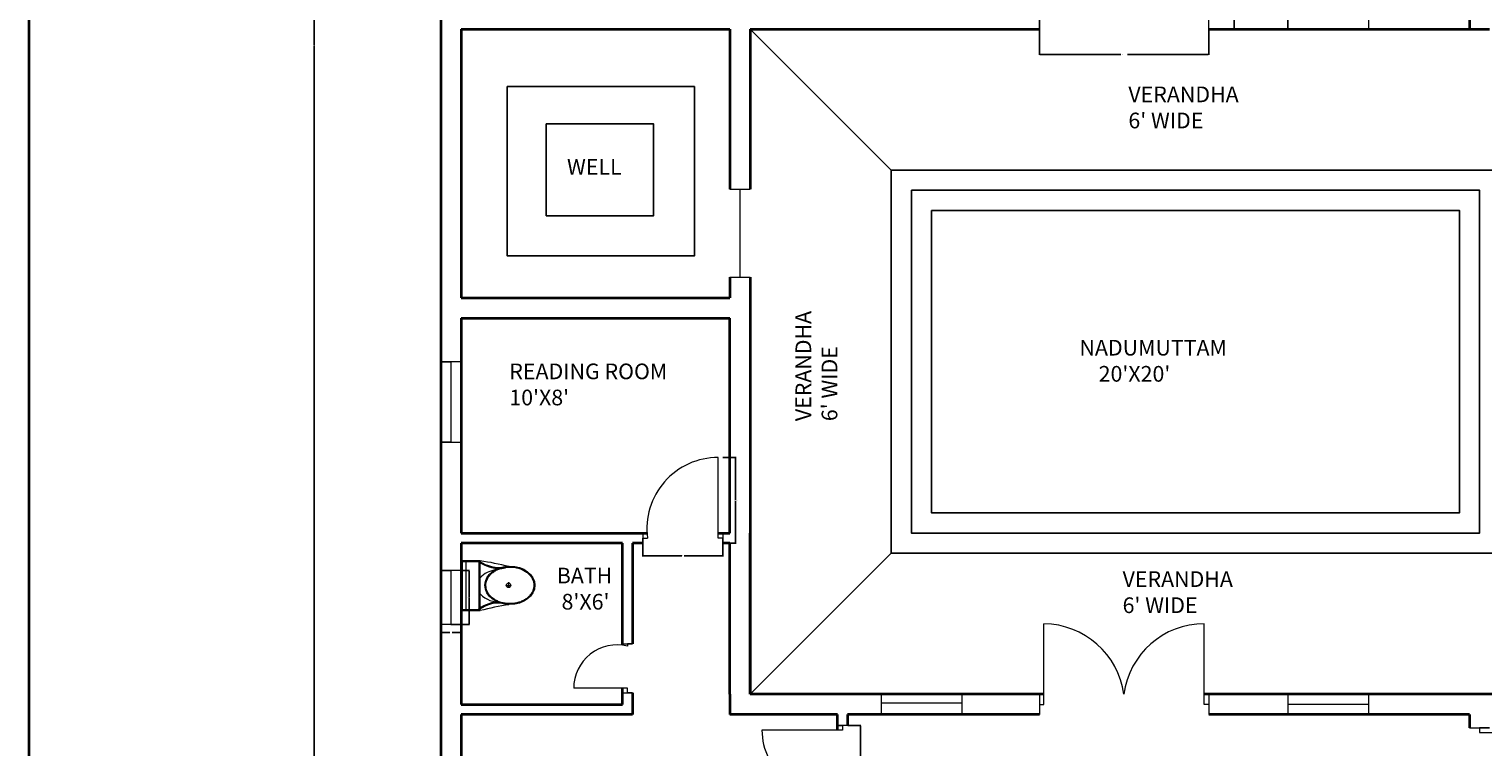
# Model space of a CAD drawing. Units: inches. Extents: x 2185 to 4426, y 1138 to 3073.
# Tile 3 of 14: x 2185 to 2834, y 1514 to 1834. Entities that reach past the tile are written whole.
import ezdxf

# ---------------------------------------------------------------- set-up
doc = ezdxf.new("R2010")
doc.units = ezdxf.units.IN
for name, color, linetype, lineweight in [('A-ANNO-DIMS', 2, 'Continuous', 18), ('A-ANNO-TTLB', 7, 'Continuous', 35), ('A-AREA-IDEN', 7, 'Continuous', 18), ('A-DOOR', 3, 'Continuous', 18), ('A-FLOR-EDGE', 7, 'Continuous', 25), ('A-FLOR-FIXT', 9, 'Continuous', 18), ('A-GLAZ', 4, 'Continuous', 18), ('A-SITE-WELL', 7, 'Continuous', 25), ('A-WALL', 7, 'Continuous', 35)]:
    doc.layers.add(name, color=color, linetype=linetype, lineweight=lineweight)
doc.styles.get("Standard").update_dxf_attribs({"font": 'arial.ttf'})
doc.dimstyles.get("Standard").update_dxf_attribs({"dimtxt": 0.18, "dimasz": 0.18, "dimexe": 0.18, "dimexo": 0.0625, "dimgap": 0.09, "dimtad": 0, "dimtih": 1, "dimtoh": 1, "dimdec": 4, "dimzin": 0, "dimdsep": 46, "dimtxsty": 'Standard', "dimcen": 0.09, "dimadec": 0, "dimazin": 0, "dimtfac": 1, "dimtdec": 4, "dimtofl": 0, "dimtmove": 0, "dimatfit": 3, "dimfxl": 1, "dimtolj": 1, "dimtzin": 0, "dimarcsym": 0})

# ---------------------------------------------------------------- blocks, each defined once
blk = doc.blocks.new('A$C31115884')
for p, q in [((283, 498), (223, 498)), ((258, 466), (258, 523)), ((0, 200), (0, 0)), ((520, 200), (0, 200)), ((10, 190), (10, 10)), ((510, 190), (10, 190)), ((510, 10), (510, 190)), ((520, 0), (520, 200)), ((510, 54), (0, 54)), ((10, 10), (510, 10)), ((0, 0), (520, 0))]:
    blk.add_line(p, q)
blk.add_circle((256, 496), 23.6)
for centre, radius, start, end in [((2778, -205), 2807, 165.4549, 171.7133), ((-295, 403), 365, 324.2091, 9.3499), ((-295, 403), 375, 324.2091, 9.3499), ((806, 403), 365, 170.6501, 215.7909), ((3237, 905), 2807, 188.2867, 194.5451), ((384, 406), 293, 190.2774, 224.1564), ((139, 406), 293, 315.8436, 2.6563), ((806, 403), 375, 179.2036, 215.7909)]:
    blk.add_arc(centre, radius, start, end)
blk.add_ellipse((256, 510), major_axis=(0, -261), ratio=0.772727)
blk.add_open_spline([(256, 259), (263, 259), (270, 260), (288, 262), (299, 265), (320, 273), (330, 278), (350, 291), (360, 299), (378, 316), (386, 326), (402, 347), (409, 358), (421, 383), (427, 395), (436, 422), (440, 436), (445, 465), (447, 480), (448, 509), (448, 524), (445, 553), (443, 568), (436, 596), (432, 610), (422, 636), (416, 649), (402, 672), (395, 683), (379, 703), (370, 712), (351, 728), (341, 735), (321, 746), (310, 751), (289, 757), (278, 759), (256, 761), (245, 761), (223, 757), (212, 754), (191, 746), (181, 741), (161, 728), (151, 720), (133, 703), (125, 693), (110, 672), (103, 660), (90, 636), (85, 623), (76, 596), (72, 582), (67, 553), (66, 538), (64, 509), (65, 494), (68, 465), (70, 450), (77, 422), (81, 408), (91, 382), (97, 370), (111, 346), (118, 335), (135, 316), (144, 307), (162, 291), (172, 284), (193, 273), (203, 269), (225, 262), (236, 260), (250, 259), (253, 259), (256, 259)], degree=3, knots=[0, 0, 0, 0, 0.110105, 0.110105, 0.285049, 0.285049, 0.459994, 0.459994, 0.634938, 0.634938, 0.809882, 0.809882, 0.984827, 0.984827, 1.159771, 1.159771, 1.334715, 1.334715, 1.50966, 1.50966, 1.684604, 1.684604, 1.859549, 1.859549, 2.034493, 2.034493, 2.209437, 2.209437, 2.384382, 2.384382, 2.559326, 2.559326, 2.73427, 2.73427, 2.909215, 2.909215, 3.084159, 3.084159, 3.259103, 3.259103, 3.434048, 3.434048, 3.608992, 3.608992, 3.783936, 3.783936, 3.958881, 3.958881, 4.133825, 4.133825, 4.30877, 4.30877, 4.483714, 4.483714, 4.658658, 4.658658, 4.833603, 4.833603, 5.008547, 5.008547, 5.183491, 5.183491, 5.358436, 5.358436, 5.53338, 5.53338, 5.708324, 5.708324, 5.883269, 5.883269, 6.058213, 6.058213, 6.233158, 6.233158, 6.283185, 6.283185, 6.283185, 6.283185])
blk = doc.blocks.new('DOOR-SGL-24-BATH-W')
for p, q in [((21.75, 21.83), (26.25, 21.83)), ((26.25, 21.83), (24, 21.83)), ((24, 21.83), (24, 20.83)), ((24, 2), (0, 2)), ((24, 0), (24, 2)), ((21.75, 0), (26.25, 0)), ((26.25, 0), (24, 0))]:
    blk.add_line(p, q)
blk.add_arc((19.38, 2), 19.38, 76.22605, 180)
blk = doc.blocks.new('DOOR-SGL-36-READING')
for p, q in [((33.62, 2.25), (33.62, 38.25)), ((0, 4.5), (0, 0)), ((0, 0), (0, 2.25)), ((0, 2.25), (2, 2.25)), ((35.62, 2.25), (33.62, 2.25)), ((35.62, 4.5), (35.62, 0)), ((35.62, 0), (35.62, 2.25))]:
    blk.add_line(p, q)
blk.add_arc((33.62, 6.36), 31.89, 90, 187.40318)
blk = doc.blocks.new('DOOR-PAIR-36-DINING')
for p, q in [((2, 4.5), (2, 40.5)), ((73.51, 4.5), (73.51, 40.5)), ((0, 9), (0, 0)), ((75.51, 0), (75.51, 9)), ((75.51, 9), (75.51, 4.5)), ((0, 0), (0, 4.5)), ((0, 4.5), (2, 4.5)), ((75.51, 4.5), (73.51, 4.5))]:
    blk.add_line(p, q)
for centre, radius, start, end in [((2, 3.7), 36.8, 8.27614, 90), ((74.14, 4.5), 36.01, 90.99344, 172.82033)]:
    blk.add_arc(centre, radius, start, end)
blk = doc.blocks.new('DOOR-SGL-36-BED-SW')
for p, q in [((36, 29.13), (0, 29.13)), ((38.25, 31.13), (33.75, 31.13)), ((33.75, 31.13), (36, 31.13)), ((36, 31.13), (36, 29.13)), ((36, 0), (36, 2)), ((33.75, 0), (38.25, 0)), ((38.25, 0), (36, 0))]:
    blk.add_line(p, q)
blk.add_arc((28.22, 29.13), 28.22, 180, 285.9925)
blk = doc.blocks.new('DOOR-PAIR-36-VERANDA')
for p, q in [((2, 4.5), (2, 40.5)), ((73.51, 4.5), (73.51, 40.5)), ((0, 9), (0, 0)), ((75.51, 9), (75.51, 0)), ((0, 4.5), (2, 4.5)), ((75.51, 4.5), (73.51, 4.5))]:
    blk.add_line(p, q)
for centre, radius, start, end in [((1.42, 3.87), 36.64, 8.05449, 89.09279), ((73.51, 4.39), 36.11, 90, 172.66346)]:
    blk.add_arc(centre, radius, start, end)
blk = doc.blocks.new('DOOR-SGL-36-BED-S')
for p, q in [((0, 31.73), (9, 31.73)), ((9, 31.73), (4.5, 31.73)), ((4.5, 31.73), (4.5, 31.73)), ((4.5, 31.73), (4.5, 29.73)), ((4.5, 29.73), (40.5, 29.73)), ((0, 0), (9, 0)), ((4.5, 0), (4.5, 2)), ((9, 0), (4.5, 0))]:
    blk.add_line(p, q)
blk.add_arc((11.82, 29.73), 28.68, 255.21093, 0)
blk = doc.blocks.new('WIN-PLAN-24IN-02')
for p, q in [((9, 24), (0, 24)), ((0, 24), (4.5, 24)), ((4.5, 24), (4.5, 0)), ((9, 0), (0, 0)), ((0, 0), (0, 0)), ((4.5, 0), (9, 0))]:
    blk.add_line(p, q)
blk = doc.blocks.new('WIN-PLAN-36IN-01')
for p, q in [((0, 9), (0, 0)), ((36, 4.5), (36, 9)), ((36, 9), (36, 0)), ((0, 0), (0, 4.5)), ((0, 4.5), (0, 4.5)), ((0, 4.5), (36, 4.5))]:
    blk.add_line(p, q)
blk = doc.blocks.new('WIN-PLAN-36IN-03')
for p, q in [((9, 36), (0, 36)), ((0, 36), (0, 36)), ((0, 36), (4.5, 36)), ((4.5, 36), (4.5, 0)), ((4.5, 0), (0, 0)), ((0, 0), (9, 0)), ((9, 0), (9, 0))]:
    blk.add_line(p, q)
blk = doc.blocks.new('WIN-PLAN-36IN-06')
for p, q in [((0, 9), (0, 0)), ((36, 9), (36, 0)), ((0, 5.12), (36, 5.12)), ((36, 5.12), (36, 5.12))]:
    blk.add_line(p, q)
blk = doc.blocks.new('WIN-PLAN-36IN-07')
for p, q in [((0, 9), (0, 0)), ((36, 9), (36, 0)), ((36, 4.5), (0, 4.5))]:
    blk.add_line(p, q)
blk = doc.blocks.new('WIN-PLAN-39IN')
for p, q in [((0, 39.26), (9, 39.26)), ((4.5, 0), (4.5, 39.26)), ((0, 0), (9, 0))]:
    blk.add_line(p, q)
blk = doc.blocks.new('WELL-PLAN')
for points in [[(0, 75.64), (83.5, 75.64), (83.5, 0), (0, 0)], [(17.44, 59), (65.29, 59), (65.29, 18), (17.44, 18)]]:
    blk.add_lwpolyline(points, close=True)
blk = doc.blocks.new('*D74')
at = {"layer": 'A-ANNO-DIMS', "color": 0, "lineweight": -2, "transparency": 16777216}
for p, q in [((2494.37, 1643.13), (2500.22, 1643.13)), ((2500.04, 1642.95), (2500.04, 1624.19)), ((2500.04, 1605.06), (2500.04, 1623.82)), ((2494.37, 1604.88), (2500.22, 1604.88))]:
    blk.add_line(p, q, dxfattribs=at)
at = {"layer": 'A-ANNO-DIMS', "color": 0, "transparency": 16777216}
for points in [[(2500.01, 1642.95), (2500.07, 1642.95), (2500.04, 1643.13)], [(2500.01, 1605.06), (2500.07, 1605.06), (2500.04, 1604.88)]]:
    blk.add_solid(points, dxfattribs=at)
at = {"layer": 'Defpoints', "color": 0, "transparency": 16777216}
for p in [(2494.31, 1643.13), (2500.04, 1643.13), (2494.31, 1604.88)]:
    blk.add_point(p, dxfattribs=at)
at = {"layer": 'A-ANNO-DIMS', "color": 0, "transparency": 16777216, "insert": (2500.04, 1624), "char_height": 0.18, "attachment_point": 5}
blk.add_mtext('\\A1;DOOR 38 TYP.', dxfattribs=at)
blk = doc.blocks.new('*D75')
at = {"layer": 'A-ANNO-DIMS', "color": 0, "lineweight": -2, "transparency": 16777216}
for p, q in [((2458.68, 1604.81), (2458.68, 1598.96)), ((2494.31, 1604.81), (2494.31, 1598.96)), ((2458.86, 1599.14), (2475.97, 1599.14)), ((2494.13, 1599.14), (2477.02, 1599.14))]:
    blk.add_line(p, q, dxfattribs=at)
at = {"layer": 'A-ANNO-DIMS', "color": 0, "transparency": 16777216}
for points in [[(2458.86, 1599.17), (2458.86, 1599.11), (2458.68, 1599.14)], [(2494.13, 1599.17), (2494.13, 1599.11), (2494.31, 1599.14)]]:
    blk.add_solid(points, dxfattribs=at)
at = {"layer": 'Defpoints', "color": 0, "transparency": 16777216}
for p in [(2458.68, 1604.88), (2494.31, 1604.88), (2494.31, 1599.14)]:
    blk.add_point(p, dxfattribs=at)
at = {"layer": 'A-ANNO-DIMS', "color": 0, "transparency": 16777216, "insert": (2476.49, 1599.14), "char_height": 0.18, "attachment_point": 5}
blk.add_mtext('\\A1;36 TYP.', dxfattribs=at)
blk = doc.blocks.new('*D76')
at = {"layer": 'A-ANNO-DIMS', "color": 0, "lineweight": -2, "transparency": 16777216}
for p, q in [((2635.64, 1834.31), (2635.64, 1822.87)), ((2711.16, 1834.31), (2711.16, 1822.87)), ((2635.82, 1823.05), (2671.91, 1823.05)), ((2710.98, 1823.05), (2674.89, 1823.05))]:
    blk.add_line(p, q, dxfattribs=at)
at = {"layer": 'A-ANNO-DIMS', "color": 0, "transparency": 16777216}
for points in [[(2635.82, 1823.08), (2635.82, 1823.02), (2635.64, 1823.05)], [(2710.98, 1823.08), (2710.98, 1823.02), (2711.16, 1823.05)]]:
    blk.add_solid(points, dxfattribs=at)
at = {"layer": 'Defpoints', "color": 0, "transparency": 16777216}
for p in [(2635.64, 1834.38), (2711.16, 1834.38), (2711.16, 1823.05)]:
    blk.add_point(p, dxfattribs=at)
at = {"layer": 'A-ANNO-DIMS', "color": 0, "transparency": 16777216, "insert": (2673.4, 1823.05), "char_height": 0.18, "attachment_point": 5}
blk.add_mtext('\\A1;DINING DOORS 76 TYP.', dxfattribs=at)
blk = doc.blocks.new('*D77')
at = {"layer": 'A-ANNO-DIMS', "color": 0, "lineweight": -2, "transparency": 16777216}
for p, q in [((2711.22, 1874.88), (2722.66, 1874.88)), ((2722.48, 1874.7), (2722.48, 1854.81)), ((2722.48, 1834.56), (2722.48, 1854.45)), ((2711.22, 1834.38), (2722.66, 1834.38))]:
    blk.add_line(p, q, dxfattribs=at)
at = {"layer": 'A-ANNO-DIMS', "color": 0, "transparency": 16777216}
for points in [[(2722.45, 1874.7), (2722.51, 1874.7), (2722.48, 1874.88)], [(2722.45, 1834.56), (2722.51, 1834.56), (2722.48, 1834.38)]]:
    blk.add_solid(points, dxfattribs=at)
at = {"layer": 'Defpoints', "color": 0, "transparency": 16777216}
for p in [(2711.16, 1874.88), (2722.48, 1874.88), (2711.16, 1834.38)]:
    blk.add_point(p, dxfattribs=at)
at = {"layer": 'A-ANNO-DIMS', "color": 0, "transparency": 16777216, "insert": (2722.48, 1854.63), "char_height": 0.18, "attachment_point": 5}
blk.add_mtext('\\A1;41 TYP.', dxfattribs=at)
blk = doc.blocks.new('*D81')
at = {"layer": 'A-ANNO-DIMS', "color": 0, "lineweight": -2, "transparency": 16777216}
for p, q in [((2550.08, 1523.44), (2555.94, 1523.44)), ((2555.76, 1523.26), (2555.76, 1507.83)), ((2555.76, 1492.05), (2555.76, 1507.47)), ((2550.08, 1491.87), (2555.94, 1491.87))]:
    blk.add_line(p, q, dxfattribs=at)
at = {"layer": 'A-ANNO-DIMS', "color": 0, "transparency": 16777216}
for points in [[(2555.73, 1523.26), (2555.79, 1523.26), (2555.76, 1523.44)], [(2555.73, 1492.05), (2555.79, 1492.05), (2555.76, 1491.87)]]:
    blk.add_solid(points, dxfattribs=at)
at = {"layer": 'Defpoints', "color": 0, "transparency": 16777216}
for p in [(2550.02, 1523.44), (2555.76, 1523.44), (2550.02, 1491.87)]:
    blk.add_point(p, dxfattribs=at)
at = {"layer": 'A-ANNO-DIMS', "color": 0, "transparency": 16777216, "insert": (2555.76, 1507.65), "char_height": 0.18, "attachment_point": 5}
blk.add_mtext('\\A1;32 TYP.', dxfattribs=at)
blk = doc.blocks.new('*D92')
at = {"layer": 'A-ANNO-DIMS', "color": 0, "lineweight": -2, "transparency": 16777216}
for p, q in [((2377.58, 1592.58), (2381.3, 1592.58)), ((2381.12, 1592.4), (2381.12, 1580.77)), ((2381.12, 1568.76), (2381.12, 1580.4)), ((2377.58, 1568.58), (2381.3, 1568.58))]:
    blk.add_line(p, q, dxfattribs=at)
at = {"layer": 'A-ANNO-DIMS', "color": 0, "transparency": 16777216}
for points in [[(2381.09, 1592.4), (2381.15, 1592.4), (2381.12, 1592.58)], [(2381.09, 1568.76), (2381.15, 1568.76), (2381.12, 1568.58)]]:
    blk.add_solid(points, dxfattribs=at)
at = {"layer": 'Defpoints', "color": 0, "transparency": 16777216}
for p in [(2377.52, 1592.58), (2381.12, 1592.58), (2377.52, 1568.58)]:
    blk.add_point(p, dxfattribs=at)
at = {"layer": 'A-ANNO-DIMS', "color": 0, "transparency": 16777216, "insert": (2381.12, 1580.58), "char_height": 0.18, "attachment_point": 5}
blk.add_mtext('\\A1;WINDOW 24 TYP.', dxfattribs=at)
blk = doc.blocks.new('*D93')
at = {"layer": 'A-ANNO-DIMS', "color": 0, "lineweight": -2, "transparency": 16777216}
for p, q in [((2368.52, 1568.52), (2368.52, 1564.8)), ((2368.7, 1564.98), (2372.56, 1564.98)), ((2377.34, 1564.98), (2373.48, 1564.98)), ((2377.52, 1568.52), (2377.52, 1564.8))]:
    blk.add_line(p, q, dxfattribs=at)
at = {"layer": 'A-ANNO-DIMS', "color": 0, "transparency": 16777216}
for points in [[(2368.7, 1565.01), (2368.7, 1564.95), (2368.52, 1564.98)], [(2377.34, 1565.01), (2377.34, 1564.95), (2377.52, 1564.98)]]:
    blk.add_solid(points, dxfattribs=at)
at = {"layer": 'Defpoints', "color": 0, "transparency": 16777216}
for p in [(2368.52, 1568.58), (2377.52, 1568.58), (2377.52, 1564.98)]:
    blk.add_point(p, dxfattribs=at)
at = {"layer": 'A-ANNO-DIMS', "color": 0, "transparency": 16777216, "insert": (2373.02, 1564.98), "char_height": 0.18, "attachment_point": 5}
blk.add_mtext('\\A1;9 TYP.', dxfattribs=at)
blk = doc.blocks.new('*D139')
at = {"layer": 'A-ANNO-DIMS', "color": 0, "lineweight": -2, "transparency": 16777216}
for p, q in [((2368.46, 2326.38), (2311.84, 2326.38)), ((2312.02, 2326.2), (2312.02, 1827.06)), ((2312.02, 1327.56), (2312.02, 1826.7)), ((2368.46, 1327.38), (2311.84, 1327.38))]:
    blk.add_line(p, q, dxfattribs=at)
at = {"layer": 'A-ANNO-DIMS', "color": 0, "transparency": 16777216}
for points in [[(2311.99, 2326.2), (2312.05, 2326.2), (2312.02, 2326.38)], [(2311.99, 1327.56), (2312.05, 1327.56), (2312.02, 1327.38)]]:
    blk.add_solid(points, dxfattribs=at)
at = {"layer": 'Defpoints', "color": 0, "transparency": 16777216}
for p in [(2312.02, 2326.38), (2368.52, 2326.38), (2368.52, 1327.38)]:
    blk.add_point(p, dxfattribs=at)
at = {"layer": 'A-ANNO-DIMS', "color": 0, "transparency": 16777216, "insert": (2312.02, 1826.88), "char_height": 0.18, "attachment_point": 5}
blk.add_mtext('\\A1;999', dxfattribs=at)

msp = doc.modelspace()

# ---------------------------------------------------------------- linework, layer by layer
at = {"layer": 'A-ANNO-TTLB'}
msp.add_lwpolyline([(2184.741, 3073.364), (4426.252, 3073.364), (4426.252, 1137.99), (2184.741, 1137.99)], close=True, dxfattribs=at)
at = {"layer": 'A-FLOR-EDGE'}
for p, q in [((2569.478, 1771.377), (2506.519, 1834.377)), ((2832.019, 1762.377), (2578.478, 1762.377)), ((2578.478, 1762.377), (2578.478, 1609.377)), ((2832.019, 1609.377), (2832.019, 1762.377)), ((2578.478, 1609.377), (2832.019, 1609.377)), ((2569.478, 1600.377), (2506.519, 1537.377))]:
    msp.add_line(p, q, dxfattribs=at)
for points in [[(2569.478, 1771.377), (2841.019, 1771.377), (2841.019, 1600.377), (2569.478, 1600.377)], [(2578.478, 1762.377), (2832.019, 1762.377), (2832.019, 1609.377), (2578.478, 1609.377)], [(2587.478, 1753.377), (2823.019, 1753.377), (2823.019, 1618.377), (2587.478, 1618.377)]]:
    msp.add_lwpolyline(points, close=True, dxfattribs=at)
at = {"layer": 'A-WALL'}
for p, q in [((2368.519, 2136.303), (2368.519, 1327.377)), ((2368.519, 2136.303), (2368.519, 1327.377)), ((2827.519, 1843.377), (2827.519, 1834.377)), ((2377.519, 1834.377), (2497.519, 1834.377)), ((2377.519, 1834.377), (2377.519, 1714.377)), ((2497.519, 1834.377), (2497.519, 1762.843)), ((2506.519, 1834.377), (2506.519, 1762.843)), ((2506.519, 1834.377), (2521.519, 1834.377)), ((2521.519, 1834.377), (2635.644, 1834.377)), ((2711.156, 1834.377), (2836.519, 1834.377)), ((2497.519, 1723.587), (2497.519, 1714.377)), ((2506.519, 1723.587), (2506.519, 1705.377)), ((2377.519, 1714.377), (2497.519, 1714.377)), ((2377.519, 1705.377), (2497.519, 1705.377)), ((2377.519, 1705.377), (2377.519, 1609.377)), ((2377.519, 1705.377), (2377.519, 1609.377)), ((2497.519, 1609.377), (2497.519, 1705.377)), ((2506.519, 1705.377), (2506.519, 1537.377)), ((2377.519, 1609.377), (2460.47, 1609.377)), ((2492.307, 1609.377), (2497.519, 1609.377)), ((2506.519, 1609.377), (2506.519, 1604.877)), ((2506.519, 1537.377), (2506.519, 1609.377)), ((2377.519, 1604.877), (2377.519, 1532.877)), ((2449.519, 1604.877), (2377.519, 1604.877)), ((2377.519, 1604.877), (2377.519, 1532.877)), ((2449.519, 1559.295), (2449.519, 1604.877)), ((2454.019, 1604.877), (2454.019, 1559.882)), ((2458.682, 1604.877), (2454.019, 1604.877)), ((2497.519, 1604.877), (2494.307, 1604.877)), ((2497.519, 1537.377), (2497.519, 1604.877)), ((2449.519, 1532.877), (2449.519, 1540.055)), ((2454.019, 1538.055), (2454.019, 1537.377)), ((2377.519, 1532.877), (2449.519, 1532.877)), ((2377.519, 1532.877), (2449.519, 1532.877)), ((2425.519, 1532.877), (2449.519, 1532.877)), ((2454.019, 1537.377), (2454.019, 1528.377)), ((2497.519, 1537.377), (2497.519, 1528.377)), ((2637.644, 1537.377), (2506.519, 1537.377)), ((2506.519, 1537.377), (2506.519, 1537.377)), ((2746.431, 1537.377), (2709.156, 1537.377)), ((2904.019, 1537.377), (2746.431, 1537.377)), ((2377.519, 1528.377), (2377.519, 1336.377)), ((2377.519, 1528.377), (2377.519, 1336.377)), ((2454.019, 1528.377), (2377.519, 1528.377)), ((2454.019, 1528.377), (2454.019, 1528.377)), ((2545.519, 1528.377), (2497.519, 1528.377)), ((2545.519, 1521.439), (2545.519, 1528.377)), ((2550.019, 1528.377), (2550.019, 1523.439)), ((2635.644, 1528.377), (2550.019, 1528.377)), ((2746.431, 1528.377), (2711.156, 1528.377)), ((2827.519, 1528.377), (2746.431, 1528.377)), ((2827.519, 1528.377), (2827.519, 1522.356))]:
    msp.add_line(p, q, dxfattribs=at)

# ---------------------------------------------------------------- block references
at = {"layer": 'A-DOOR'}
for name, p in [('DOOR-PAIR-36-DINING', (2635.644, 1834.377)), ('DOOR-SGL-36-READING', (2458.682, 1604.877)), ('DOOR-PAIR-36-VERANDA', (2635.644, 1528.377)), ('DOOR-SGL-24-BATH-W', (2427.769, 1538.055)), ('DOOR-SGL-36-BED-SW', (2511.769, 1492.307)), ('DOOR-SGL-36-BED-S', (2827.519, 1490.627))]:
    msp.add_blockref(name, p, dxfattribs=at)
at = {"layer": 'A-FLOR-FIXT', "xscale": 0.0427196977339482, "yscale": 0.0427196977339482, "zscale": 0.0427196977339482, "rotation": 270}
msp.add_blockref('A$C31115884', (2377.519, 1596.969), dxfattribs=at)
at = {"layer": 'A-GLAZ'}
for name, p in [('WIN-PLAN-36IN-01', (2746.431, 1834.377)), ('WIN-PLAN-39IN', (2497.519, 1723.587)), ('WIN-PLAN-36IN-03', (2368.519, 1649.883)), ('WIN-PLAN-24IN-02', (2368.519, 1568.585)), ('WIN-PLAN-36IN-06', (2565.039, 1528.377)), ('WIN-PLAN-36IN-07', (2746.431, 1528.377))]:
    msp.add_blockref(name, p, dxfattribs=at)
at = {"layer": 'A-SITE-WELL'}
msp.add_blockref('WELL-PLAN', (2398.119, 1733.064), dxfattribs=at)

# ---------------------------------------------------------------- texts
at = {"layer": 'A-AREA-IDEN', "char_height": 7, "attachment_point": 1}
for s, width, insert in [("VERANDHA\\P6' WIDE", 210.80817, (2675.304, 1808.725)), ('WELL', 103.13785, (2424.797, 1776.364)), ("NADUMUTTAM\\P    20'X20'", 247.49347, (2653.483, 1695.626)), ("READING ROOM\\P10'X8'", 85.98877, (2399.056, 1685.053)), ("BATH\\P 8'X6'", 202.02529, (2420.234, 1593.883)), ("VERANDHA\\P6' WIDE", 210.80817, (2672.724, 1592.314))]:
    msp.add_mtext_dynamic_manual_height_columns(s, width=width, gutter_width=12.5, heights=[0], dxfattribs=dict(at, insert=insert))
at = {"layer": 'A-AREA-IDEN', "insert": (2526.757, 1659.313), "char_height": 7, "attachment_point": 1, "rotation": 90}
msp.add_mtext_dynamic_manual_height_columns("VERANDHA\\P6' WIDE", width=210.80817, gutter_width=12.5, heights=[0], dxfattribs=at)

# ---------------------------------------------------------------- dimensions: what is measured, and where the dimension line sits
at = {"layer": 'A-ANNO-DIMS'}
dim = msp.add_linear_dim(base=(2312.019, 2326.377), p1=(2368.519, 1327.377), p2=(2368.519, 2326.377), angle=90, dimstyle='Standard', override={"dimdec": 0, "dimlfac": 1, "dimrnd": 0, "dimzin": 0, "dimdsep": 46, "dimlunit": 2}, dxfattribs=at)
dim.commit()
dim.dimension.update_dxf_attribs({"geometry": '*D139', "text_midpoint": (2312.019, 1826.877)})
for base, p1, p2, text, picture, middle in [((2722.483242552, 1874.876947079), (2711.156398771, 1834.376947079), (2711.156398771, 1874.876947079), '<> TYP.', '*D77', (2722.483242552, 1854.626947079)), ((2500.044, 1643.127), (2494.307, 1604.877), (2494.307, 1643.127), 'DOOR <> TYP.', '*D74', (2500.044, 1624.002)), ((2381.119, 1592.585), (2377.519, 1568.585), (2377.519, 1592.585), 'WINDOW <> TYP.', '*D92', (2381.119, 1580.585)), ((2555.757, 1523.439), (2550.019, 1491.866), (2550.019, 1523.439), '<> TYP.', '*D81', (2555.757, 1507.652))]:
    dim = msp.add_linear_dim(base=base, p1=p1, p2=p2, angle=90, text=text, dimstyle='Standard', override={"dimdec": 0, "dimlfac": 1, "dimrnd": 0, "dimzin": 0, "dimdsep": 46, "dimlunit": 2}, dxfattribs=at)
    dim.commit()
    dim.dimension.update_dxf_attribs({"geometry": picture, "text_midpoint": middle})
for base, p1, p2, text, picture, middle in [((2711.156, 1823.05), (2635.644, 1834.377), (2711.156, 1834.377), 'DINING DOORS <> TYP.', '*D76', (2673.4, 1823.05)), ((2494.307, 1599.139), (2458.682, 1604.877), (2494.307, 1604.877), '<> TYP.', '*D75', (2476.494, 1599.139)), ((2377.519, 1564.985), (2368.519, 1568.585), (2377.519, 1568.585), '<> TYP.', '*D93', (2373.019, 1564.985))]:
    dim = msp.add_linear_dim(base=base, p1=p1, p2=p2, text=text, dimstyle='Standard', override={"dimdec": 0, "dimlfac": 1, "dimrnd": 0, "dimzin": 0, "dimdsep": 46, "dimlunit": 2}, dxfattribs=at)
    dim.commit()
    dim.dimension.update_dxf_attribs({"geometry": picture, "text_midpoint": middle})

doc.saveas('drawing.dxf')
